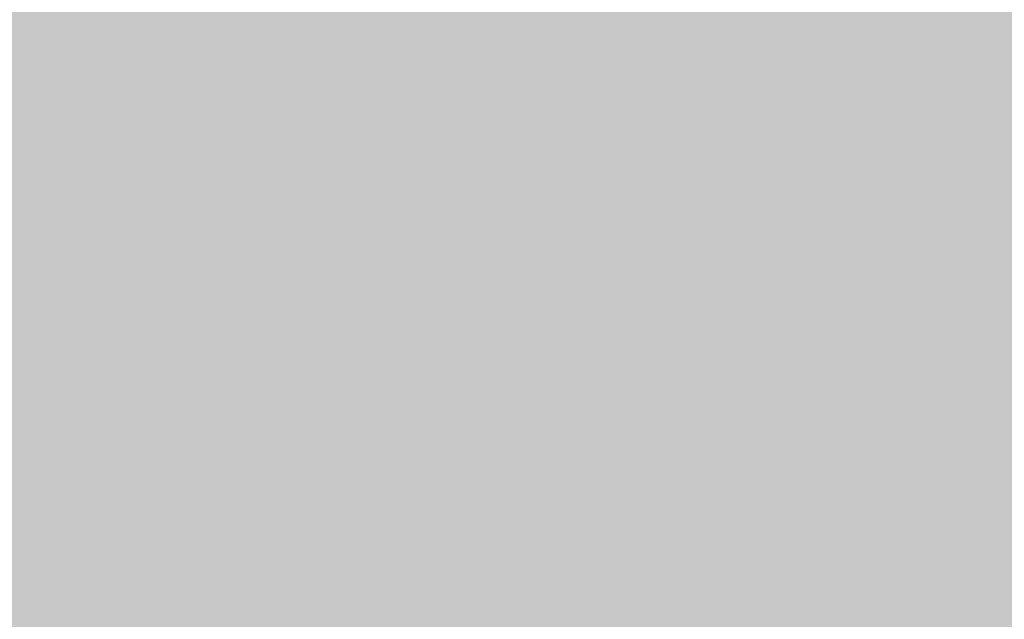
# Model space of a CAD drawing. Units: feet. Extents: x 3168 to 4724, y 827 to 1477.
# Tile 61 of 256: x 3273.145496 to 3273.147847, y 1099.01485 to 1099.016281. Entities that reach past the tile are written whole.
import ezdxf

# ---------------------------------------------------------------- set-up
doc = ezdxf.new("R2010")
doc.units = ezdxf.units.FT
doc.layers.add('A-ELEV', color=7, linetype='Continuous', lineweight=35)
doc.layers.add('A-ELEV-PATT', color=8, linetype='Continuous', lineweight=13)

msp = doc.modelspace()

# ---------------------------------------------------------------- hatches: boundary and pattern name
at = {"layer": 'A-ELEV-PATT'}
h = msp.add_hatch(color=256, dxfattribs=at)
h.dxf.hatch_style = 1
edge = h.paths.add_edge_path()
edge.add_ellipse((3552.9057615, 979.2201412), major_axis=(36.7449243, 0), ratio=0.4848484848, start_angle=0, end_angle=360)
edge = h.paths.add_edge_path()
edge.add_ellipse((3559.8916366, 929.2522824), major_axis=(36.7449243, 0), ratio=0.4848484848, start_angle=0, end_angle=360)
edge = h.paths.add_edge_path()
edge.add_line((3299.3168105, 1198.606081), (3479.9167135, 1198.606081))
edge.add_line((3479.9167135, 1198.606081), (3479.9167135, 1209.8685704))
edge.add_spline(control_points=[(3479.9167135, 1209.8685704), (3464.3011571, 1209.8685704), (3448.6856007, 1209.8685704), (3410.949139, 1209.8685704), (3388.8282339, 1209.8685704), (3355.6468761, 1209.8685704), (3344.5864235, 1209.8685704), (3327.9957446, 1209.8685704), (3322.4655183, 1209.8685704), (3314.1701788, 1209.8685704), (3311.4050657, 1209.8685704), (3307.257396, 1209.8685704), (3305.8748394, 1209.8685704), (3303.8010045, 1209.8685704), (3303.1097262, 1209.8685704), (3302.0728088, 1209.8685704), (3301.7271697, 1209.8685704), (3301.2087109, 1209.8685704), (3301.0358914, 1209.8685704), (3300.776662, 1209.8685704), (3300.6902522, 1209.8685704), (3300.5606376, 1209.8685704), (3300.5174327, 1209.8685704), (3300.4526253, 1209.8685704), (3300.4310229, 1209.8685704), (3300.3986192, 1209.8685704), (3300.387818, 1209.8685704), (3300.3662155, 1209.8685704), (3300.3456757, 1209.8685704), (3300.3455476, 1209.8685704), (3300.345505, 1209.8685704), (3300.3433041, 1209.8685704), (3300.341146, 1209.8685707), (3300.337909, 1209.8685714), (3300.33683, 1209.8685718), (3300.3339422, 1209.8685728), (3300.3321334, 1209.8685736), (3300.3255154, 1209.8685773), (3300.3207065, 1209.8685812), (3300.3109248, 1209.8685917), (3300.305952, 1209.8685984), (3300.2905113, 1209.8686233), (3300.2800452, 1209.8686461), (3300.2324255, 1209.868777), (3300.1952979, 1209.868954), (3299.9510684, 1209.8706077), (3299.7448244, 1209.8743259), (3299.4368271, 1209.8832566), (3299.3343894, 1209.8867924), (3299.181079, 1209.8929197), (3299.1300333, 1209.8950994), (3298.6522171, 1209.9168011), (3298.2294605, 1209.9457176), (3297.6016312, 1210.0023671), (3297.3934043, 1210.0234637), (3297.082652, 1210.058309), (3296.9793324, 1210.0704575), (3296.2929541, 1210.1548606), (3295.7181475, 1210.2433556), (3294.8687167, 1210.3988504), (3294.5876997, 1210.4544779), (3294.1693407, 1210.5433488), (3294.0304153, 1210.5738777), (3291.7071487, 1211.1012), (3289.6535901, 1211.8134353), (3285.7762586, 1213.5639876), (3283.9514101, 1214.6034778), (3280.512159, 1216.9800798), (3278.8972407, 1218.3175918), (3276.3799143, 1220.829489), (3275.4160415, 1221.9177379), (3274.0393421, 1223.7076996), (3273.5810428, 1224.3495346), (3273.1432283, 1225.0163162)], knot_values=[39.119033, 39.119033, 39.119033, 39.119033, 39.286353, 39.286353, 39.523379, 39.523379, 39.641892, 39.641892, 39.701148, 39.701148, 39.730777, 39.730777, 39.745591, 39.745591, 39.752998, 39.752998, 39.756701, 39.756701, 39.758553, 39.758553, 39.759479, 39.759479, 39.759942, 39.759942, 39.760173, 39.760173, 39.760289, 39.760289, 39.760405, 39.760405, 39.760463, 39.760463, 39.763389, 39.763389, 39.764851, 39.764851, 39.767304, 39.767304, 39.773825, 39.773825, 39.78057, 39.78057, 39.79477, 39.79477, 39.845194, 39.845194, 40.126715, 40.126715, 40.267476, 40.267476, 40.337856, 40.337856, 40.927023, 40.927023, 41.221606, 41.221606, 41.368898, 41.368898, 42.202622, 42.202622, 42.619485, 42.619485, 42.827916, 42.827916, 46.118323, 46.118323, 49.408731, 49.408731, 52.699139, 52.699139, 54.927489, 54.927489, 56.104228, 56.104228, 56.104228, 56.104228], weights=[1, 1, 1, 1, 1, 1, 1, 1, 1, 1, 1, 1, 1, 1, 1, 1, 1, 1, 1, 1, 1, 1, 1, 1, 1, 1, 1, 1, 1, 1, 1, 1, 1, 1, 1, 1, 1, 1, 1, 1, 1, 1, 1, 1, 1, 1, 1, 1, 1, 1, 1, 1, 1, 1, 1, 1, 1, 1, 1, 1, 1, 1, 1, 1, 1, 1, 1, 1, 1, 1, 1, 1, 1, 1], degree=3, periodic=0)
edge.add_line((3273.1432283, 1225.0163162), (3273.1432283, 1099.0163162))
edge.add_line((3273.1432283, 1099.0163162), (3299.3168105, 1099.0163162))
edge.add_line((3299.3168105, 1099.0163162), (3299.3168105, 1198.606081))
edge = h.paths.add_edge_path()
edge.add_line((3304.7584434, 1324.15806), (3479.9167135, 1324.15806))
edge.add_line((3479.9167135, 1324.15806), (3479.9167135, 1335.7146184))
edge.add_line((3479.9167135, 1335.7146184), (3269.1616284, 1335.7146184))
edge.add_spline(control_points=[(3269.1616284, 1335.7146184), (3264.0242315, 1335.7146184), (3258.364118, 1328.9581888), (3259.2643109, 1323.9002743)], knot_values=[0, 0, 0, 0, 15.412191, 15.412191, 15.412191, 15.412191], degree=3, periodic=0)
edge.add_line((3259.2643109, 1323.9002743), (3265.5168487, 1288.7691348))
edge.add_line((3265.5168487, 1288.7691348), (3275.2651026, 1261.5456259))
edge.add_line((3275.2651026, 1261.5456259), (3304.7584434, 1261.5456259))
edge.add_line((3304.7584434, 1261.5456259), (3304.7584434, 1324.15806))
h = msp.add_hatch(color=256, dxfattribs=at)
h.dxf.hatch_style = 1
h.paths.add_polyline_path([(3384.5252473, 1099.0163162), (3335.0291678, 1099.0163162), (3299.3168105, 1099.0163162), (3273.1432283, 1099.0163162), (3217.5653642, 1099.0163162), (3168.0692847, 827.1162598), (3335.0291678, 827.1162598)])

# ---------------------------------------------------------------- linework, layer by layer
at = {"layer": 'A-ELEV'}
msp.add_open_spline([(3808.5202001, 1099.0163162), (3808.5202001, 1141.413235), (3808.5202001, 1183.8101539), (3808.5202001, 1226.6353244), (3808.5202001, 1227.0635761), (3808.5202001, 1227.4918279), (3811.491871, 1248.9946729), (3814.463542, 1270.497518), (3817.4652299, 1292.2175635), (3817.4952467, 1292.434764), (3817.5252636, 1292.6519644), (3817.5728014, 1310.1067483), (3817.6203393, 1327.5615322), (3817.6678771, 1345.0163162), (3817.6678771, 1345.4579619), (3817.6678771, 1345.8996077), (3817.6678771, 1346.4560466), (3817.6678771, 1346.5708398), (3817.6678771, 1346.7528874), (3817.6678771, 1346.8201418), (3817.6678771, 1346.9348705), (3817.6678771, 1346.9823447), (3817.6678771, 1347.0385872), (3817.6678771, 1347.0473556), (3817.6678771, 1347.0736607), (3817.667877, 1347.0593025), (3817.6678766, 1347.0615455), (3817.6678764, 1347.0626669), (3817.6678754, 1347.0660311), (3817.6678743, 1347.0682738), (3817.6678701, 1347.0750012), (3817.667866, 1347.0794856), (3817.6678493, 1347.0929368), (3817.6678325, 1347.1019019), (3817.6677657, 1347.1287896), (3817.6676988, 1347.1467049), (3817.6674317, 1347.2004211), (3817.6671649, 1347.2361922), (3817.6661003, 1347.3433849), (3817.6650383, 1347.4146859), (3817.6608124, 1347.6280949), (3817.6566084, 1347.7697085), (3817.6399698, 1348.1924868), (3817.6235091, 1348.4715855), (3817.5590944, 1349.3000666), (3817.4961208, 1349.8405878), (3817.2554319, 1351.4241561), (3817.0263177, 1352.4287852), (3816.3068713, 1354.8889138), (3815.7437452, 1356.2687272), (3814.4639586, 1358.8192105), (3813.7464132, 1359.9909676), (3812.1958378, 1362.1723433), (3811.3622453, 1363.1821237), (3809.5888357, 1365.0690087), (3808.6488164, 1365.9461052), (3806.6542623, 1367.5796162), (3805.5997024, 1368.336154), (3803.3528906, 1369.7223272), (3802.1605354, 1370.352386), (3799.6008131, 1371.4535864), (3798.2326878, 1371.9254812), (3795.2800838, 1372.6346239), (3793.6931479, 1372.8720685), (3791.8694413, 1372.9264797), (3791.7408615, 1372.9292203), (3791.3533713, 1372.9341014), (3791.0927074, 1372.9329013), (3790.3041163, 1372.9150676), (3789.7695426, 1372.8841946), (3789.20919, 1372.8302363), (3789.1906217, 1372.8284241), (3789.1348916, 1372.8229123), (3789.097705, 1372.8191375), (3789.0484446, 1372.8140077), (3789.0364001, 1372.8127432), (3789.0002562, 1372.808918), (3788.9761468, 1372.8063255), (3788.9494049, 1372.8034042), (3788.9467858, 1372.8031177), (3788.9425667, 1372.8026552), (3788.9409669, 1372.8024797), (3788.9385718, 1372.8022166), (3788.9377765, 1372.8021292), (3788.9353908, 1372.8018669), (3788.8675349, 1372.7944024), (3788.7568665, 1372.7822285), (3788.7015323, 1372.7761415), (3788.5355297, 1372.7578805), (3788.4248612, 1372.7457065), (3788.092856, 1372.7091846), (3787.8715192, 1372.6848366), (3787.2075086, 1372.6117927), (3786.764835, 1372.5630968), (3785.436814, 1372.417009), (3784.5514666, 1372.3196171), (3781.8954246, 1372.0274416), (3780.1247299, 1371.8326579), (3774.8126458, 1371.2483067), (3771.2712564, 1370.8587393), (3760.6470883, 1369.6900371), (3753.5643095, 1368.9109022), (3732.3159732, 1366.5734977), (3718.1504157, 1365.015228), (3694.0067577, 1362.3593262), (3684.0286573, 1361.2616941), (3674.0505568, 1360.1640619), (3664.6006617, 1360.1640619), (3655.1507666, 1360.1640619), (3626.8010812, 1360.1640619), (3607.9012909, 1360.1640619), (3551.2019201, 1360.1640619), (3513.4023395, 1360.1640619), (3467.7251817, 1360.1640619), (3459.8476045, 1360.1640619), (3436.2148727, 1360.1640619), (3420.4597182, 1360.1640619), (3373.1942547, 1360.1640619), (3341.6839457, 1360.1640619), (3302.8481616, 1360.1640619), (3295.5226865, 1360.1640619), (3286.0382916, 1360.1640619), (3283.8793719, 1360.1640619), (3277.4026128, 1360.1640619), (3273.0847733, 1360.1640619), (3267.7328511, 1360.1640619), (3266.6987684, 1360.1640619), (3263.5965201, 1360.1640619), (3261.5283546, 1360.1640619), (3259.2369429, 1360.1640619), (3259.0136967, 1360.1640619), (3258.3439582, 1360.1640619), (3257.8974658, 1360.1640619), (3257.4309979, 1360.1640619), (3257.4110224, 1360.1640619), (3257.3705735, 1360.1640619), (3257.3754695, 1360.1640619), (3257.3745975, 1360.1640619), (3257.3739371, 1360.1640618), (3257.3719559, 1360.1640616), (3257.3706351, 1360.1640613), (3257.366673, 1360.16406), (3257.3640318, 1360.1640586), (3257.3561088, 1360.1640529), (3257.3508277, 1360.1640469), (3257.3349869, 1360.1640226), (3257.3244299, 1360.163998), (3257.2927692, 1360.1638987), (3257.2716761, 1360.1637987), (3257.208439, 1360.1633975), (3257.1663373, 1360.1629953), (3257.0402058, 1360.1613882), (3256.9563493, 1360.1597827), (3256.705504, 1360.1533932), (3256.53924, 1360.1470361), (3256.0435702, 1360.1219156), (3255.717296, 1360.0971018), (3254.7524458, 1360.0004808), (3254.1279679, 1359.906513), (3252.1800666, 1359.5253322), (3250.9415739, 1359.1439911), (3248.6701751, 1358.2432905), (3247.6357388, 1357.7238339), (3245.7326321, 1356.6034712), (3244.8633884, 1356.0020595), (3243.2531076, 1354.7428655), (3242.511972, 1354.0847309), (3240.7510518, 1352.3447812), (3239.8009609, 1351.229574), (3238.0877694, 1348.8724402), (3237.3246853, 1347.6303552), (3235.9825098, 1344.9716321), (3235.4022051, 1343.554907), (3234.5910812, 1340.8154577), (3234.3108819, 1339.5435498), (3233.9764902, 1336.8025605), (3233.9221126, 1335.3308771), (3234.1489156, 1332.5912693), (3234.3495287, 1331.3672011), (3234.7198926, 1329.9993668), (3234.7524228, 1329.8833616), (3234.853619, 1329.5347966), (3234.9258923, 1329.301685), (3235.0248359, 1329.0025524), (3235.0469235, 1328.936928), (3235.0776388, 1328.8472393), (3235.0859239, 1328.8231979), (3235.1109389, 1328.7510642), (3235.1278282, 1328.7029624), (3235.1479919, 1328.6462418), (3235.1510592, 1328.6376324), (3235.1560959, 1328.6235265), (3235.1580611, 1328.6180301), (3235.1602094, 1328.6120302), (3235.1656119, 1328.596943), (3235.1800989, 1328.556486), (3235.190263, 1328.5281009), (3235.2207556, 1328.4429457), (3235.241084, 1328.3861755), (3235.3020692, 1328.215865), (3235.3427259, 1328.1023247), (3235.4646962, 1327.7617038), (3235.5460097, 1327.5346232), (3235.7899503, 1326.8533813), (3235.9525774, 1326.39922), (3236.4404586, 1325.0367362), (3236.7657127, 1324.1284137), (3237.7414751, 1321.4034462), (3238.3919833, 1319.5868011), (3240.3435081, 1314.136866), (3241.6445245, 1310.503576), (3245.547574, 1299.6037058), (3248.149607, 1292.3371257), (3255.955706, 1270.5373853), (3261.1597719, 1256.004225), (3267.3876177, 1238.6120011), (3268.4113975, 1235.7529374), (3269.5103781, 1232.6838639), (3269.5855789, 1232.473854), (3269.7066118, 1232.1358507), (3269.752444, 1232.0078573), (3269.8273289, 1231.7987296), (3269.8563817, 1231.7175953), (3269.9063247, 1231.5781217), (3269.927215, 1231.5197823), (3269.9724682, 1231.3934057), (3269.9968311, 1231.3253685), (3270.0265026, 1231.2425062), (3270.0318112, 1231.2276812), (3270.0402823, 1231.2040243), (3270.0392242, 1231.2069792), (3270.0393595, 1231.2066014), (3270.0394271, 1231.2064125), (3270.0396301, 1231.2058458), (3270.0397654, 1231.205468), (3270.0401713, 1231.2043346), (3270.040442, 1231.2035791), (3270.041254, 1231.2013125), (3270.0417955, 1231.1998016), (3270.0434203, 1231.195269), (3270.044504, 1231.1922477), (3270.0477563, 1231.1831849), (3270.0499263, 1231.1771446), (3270.0564418, 1231.1590283), (3270.0607927, 1231.146957), (3270.0738674, 1231.1107614), (3270.0826128, 1231.0866558), (3270.1089357, 1231.0144129), (3270.1265997, 1230.9663498), (3270.1799341, 1230.8224568), (3270.2159467, 1230.7269233), (3270.3253234, 1230.4415078), (3270.4000257, 1230.2528107), (3270.6292491, 1229.6914436), (3270.7888829, 1229.3235005), (3271.2864875, 1228.2383194), (3271.6430996, 1227.5397546), (3272.7758592, 1225.515277), (3273.6141694, 1224.2605021), (3275.4160415, 1221.9177379), (3276.3799143, 1220.829489), (3278.8972407, 1218.3175918), (3280.512159, 1216.9800798), (3283.9514101, 1214.6034778), (3285.7762586, 1213.5639876), (3289.6535901, 1211.8134353), (3291.7071487, 1211.1012), (3294.0304153, 1210.5738777), (3294.1693407, 1210.5433488), (3294.5876997, 1210.4544779), (3294.8687167, 1210.3988504), (3295.7181475, 1210.2433556), (3296.2929541, 1210.1548606), (3296.9793324, 1210.0704575), (3297.082652, 1210.058309), (3297.3934043, 1210.0234637), (3297.6016312, 1210.0023671), (3298.2294605, 1209.9457176), (3298.6522171, 1209.9168011), (3299.1300333, 1209.8950994), (3299.181079, 1209.8929197), (3299.3343894, 1209.8867924), (3299.4368271, 1209.8832566), (3299.7448244, 1209.8743259), (3299.9510684, 1209.8706077), (3300.1952979, 1209.868954), (3300.2324255, 1209.868777), (3300.2800452, 1209.8686461), (3300.2905113, 1209.8686233), (3300.305952, 1209.8685984), (3300.3109248, 1209.8685917), (3300.3207065, 1209.8685812), (3300.3255154, 1209.8685773), (3300.3321334, 1209.8685736), (3300.3339422, 1209.8685728), (3300.33683, 1209.8685718), (3300.337909, 1209.8685714), (3300.341146, 1209.8685707), (3300.3433041, 1209.8685704), (3300.345505, 1209.8685704), (3300.3455476, 1209.8685704), (3300.3456757, 1209.8685704), (3300.3662155, 1209.8685704), (3300.387818, 1209.8685704), (3300.3986192, 1209.8685704), (3300.4310229, 1209.8685704), (3300.4526253, 1209.8685704), (3300.5174327, 1209.8685704), (3300.5606376, 1209.8685704), (3300.6902522, 1209.8685704), (3300.776662, 1209.8685704), (3301.0358914, 1209.8685704), (3301.2087109, 1209.8685704), (3301.7271697, 1209.8685704), (3302.0728088, 1209.8685704), (3303.1097262, 1209.8685704), (3303.8010045, 1209.8685704), (3305.8748394, 1209.8685704), (3307.257396, 1209.8685704), (3311.4050657, 1209.8685704), (3314.1701788, 1209.8685704), (3322.4655183, 1209.8685704), (3327.9957446, 1209.8685704), (3344.5864235, 1209.8685704), (3355.6468761, 1209.8685704), (3388.8282339, 1209.8685704), (3410.949139, 1209.8685704), (3477.3118546, 1209.8685704), (3521.553665, 1209.8685704), (3566.8361836, 1209.8685704), (3567.8768919, 1209.8685704), (3570.9990167, 1209.8685704), (3573.0804332, 1209.8685704), (3575.7813964, 1209.8685704), (3576.4009432, 1209.8685704), (3577.2958211, 1209.8685704), (3577.5711523, 1209.8685704), (3578.3971458, 1209.8685704), (3578.9478081, 1209.8685704), (3579.7564907, 1209.8685704), (3580.0145108, 1209.8685704), (3580.3427367, 1209.8685704), (3580.3268649, 1209.8685704), (3580.3271702, 1209.8685704), (3580.3273229, 1209.8685704), (3580.3277809, 1209.8685704), (3580.3280863, 1209.8685704), (3580.3290024, 1209.8685703), (3580.3296132, 1209.8685702), (3580.3314455, 1209.8685699), (3580.332667, 1209.8685697), (3580.336332, 1209.8685685), (3580.3387755, 1209.8685674), (3580.3461066, 1209.8685629), (3580.350995, 1209.8685584), (3580.3656627, 1209.8685402), (3580.3754446, 1209.868522), (3580.4048012, 1209.8684493), (3580.4243863, 1209.8683764), (3580.4831833, 1209.8680848), (3580.5224371, 1209.8677929), (3580.6403612, 1209.8666242), (3580.7191947, 1209.8654543), (3580.9563152, 1209.8607663), (3581.1152222, 1209.85607), (3581.5941635, 1209.8372298), (3581.9164188, 1209.8183314), (3582.8899466, 1209.7424284), (3583.547986, 1209.6661692), (3585.5318268, 1209.3606172), (3586.8672159, 1209.0538859), (3589.4715454, 1208.2524717), (3590.7402412, 1207.7578521), (3591.9954511, 1207.1588024), (3592.057809, 1207.1287398), (3592.2442418, 1207.0379536), (3592.3676757, 1206.9766317), (3592.73528, 1206.7903591), (3592.9767518, 1206.663101), (3593.2445387, 1206.5164414), (3593.2747313, 1206.4998248), (3593.3651153, 1206.4498388), (3593.4251129, 1206.4163333), (3593.6043138, 1206.3152851), (3593.7227254, 1206.2472105), (3593.8572122, 1206.1683978), (3593.8743621, 1206.1583193), (3593.925741, 1206.1280407), (3593.9598989, 1206.1077976), (3594.0620855, 1206.0468991), (3594.1298272, 1206.0060745), (3594.2084359, 1205.9581709), (3594.2196829, 1205.9513043), (3594.253391, 1205.9306863), (3594.2758193, 1205.9169166), (3594.3429716, 1205.8755358), (3594.3875633, 1205.8478526), (3594.4336161, 1205.8190499), (3594.4352559, 1205.818024), (3594.4401746, 1205.8149461), (3594.4434527, 1205.8128936), (3594.4471229, 1205.8105944), (3594.4475159, 1205.8103482), (3594.4486949, 1205.8096095), (3594.4494808, 1205.8091171), (3594.4503663, 1205.8085621), (3594.4504658, 1205.8084998), (3594.4506003, 1205.8084155), (3594.4673993, 1205.7978872), (3594.4932689, 1205.7816741), (3594.5062037, 1205.7735675), (3594.5450081, 1205.7492479), (3594.5708778, 1205.7330348), (3594.6484866, 1205.6843956), (3594.7002258, 1205.6519694), (3594.8554436, 1205.5546909), (3594.958922, 1205.4898386), (3595.2693574, 1205.2952816), (3595.4763144, 1205.1655769), (3596.0971852, 1204.7764629), (3596.5110991, 1204.5170536), (3597.7528407, 1203.7388256), (3598.5806685, 1203.220007), (3601.0641518, 1201.663551), (3602.7198073, 1200.6259137), (3607.686774, 1197.5130018), (3610.998085, 1195.4377272), (3620.9320182, 1189.2119034), (3627.5546404, 1185.0613542), (3647.4225068, 1172.6097066), (3660.6677511, 1164.3086082), (3700.403484, 1139.405313), (3726.8939725, 1122.8031161), (3757.2057154, 1103.8060516), (3761.0269697, 1101.4111839), (3764.848224, 1099.0163162), (3745.3282713, 1099.0163162), (3725.8083186, 1099.0163162), (3706.288366, 1099.0163162), (3706.288366, 1108.4532371), (3706.288366, 1117.890158), (3706.288366, 1127.3270789), (3710.7507544, 1127.3270789), (3715.2131428, 1127.3270789), (3719.6755312, 1127.3270789)], degree=3, knots=[0, 0, 0, 0, 0.982037, 0.982037, 0.991957, 0.991957, 0.991957, 1.966522, 1.966522, 1.976367, 1.976367, 1.976367, 2.976367, 2.976367, 2.976367, 3.00169, 3.00169, 3.008272, 3.008272, 3.012129, 3.012129, 3.014851, 3.014851, 3.015353, 3.015353, 3.016359, 3.016359, 3.017365, 3.017365, 3.019376, 3.019376, 3.023398, 3.023398, 3.031442, 3.031442, 3.047531, 3.047531, 3.079708, 3.079708, 3.144063, 3.144063, 3.272772, 3.272772, 3.53019, 3.53019, 4.045026, 4.045026, 5.074698, 5.074698, 6.700878, 6.700878, 8.327058, 8.327058, 9.953238, 9.953238, 11.579418, 11.579418, 13.205598, 13.205598, 14.831778, 14.831778, 16.457958, 16.457958, 18.084138, 18.084138, 18.206872, 18.206872, 18.45234, 18.45234, 18.943275, 18.943275, 18.960093, 18.960093, 18.993729, 18.993729, 19.00461, 19.00461, 19.026374, 19.026374, 19.028737, 19.028737, 19.03018, 19.03018, 19.030897, 19.030897, 19.032332, 19.032332, 19.033766, 19.033766, 19.036636, 19.036636, 19.042374, 19.042374, 19.053851, 19.053851, 19.076805, 19.076805, 19.122714, 19.122714, 19.21453, 19.21453, 19.398163, 19.398163, 19.765429, 19.765429, 20.024128, 20.024128, 20.024128, 20.092031, 20.092031, 20.227836, 20.227836, 20.499446, 20.499446, 20.556051, 20.556051, 20.66926, 20.66926, 20.895678, 20.895678, 20.948316, 20.948316, 20.963829, 20.963829, 20.994855, 20.994855, 21.002285, 21.002285, 21.017146, 21.017146, 21.01875, 21.01875, 21.021959, 21.021959, 21.022102, 21.022102, 21.022249, 21.022249, 21.022708, 21.022708, 21.023627, 21.023627, 21.025464, 21.025464, 21.029138, 21.029138, 21.036486, 21.036486, 21.051183, 21.051183, 21.080575, 21.080575, 21.139361, 21.139361, 21.256932, 21.256932, 21.492073, 21.492073, 21.962356, 21.962356, 23.01002, 23.01002, 24.057684, 24.057684, 25.105348, 25.105348, 26.153011, 26.153011, 27.776787, 27.776787, 29.400562, 29.400562, 31.024337, 31.024337, 32.278801, 32.278801, 33.533265, 33.533265, 34.467568, 34.467568, 34.553971, 34.553971, 34.726776, 34.726776, 34.775309, 34.775309, 34.793079, 34.793079, 34.82862, 34.82862, 34.834979, 34.834979, 34.839039, 34.839039, 34.839411, 34.839411, 34.840285, 34.840285, 34.842034, 34.842034, 34.845531, 34.845531, 34.852525, 34.852525, 34.866512, 34.866512, 34.894488, 34.894488, 34.950439, 34.950439, 35.062342, 35.062342, 35.286147, 35.286147, 35.733758, 35.733758, 35.821815, 35.821815, 35.828283, 35.828283, 35.832225, 35.832225, 35.834724, 35.834724, 35.836521, 35.836521, 35.838617, 35.838617, 35.839073, 35.839073, 35.839345, 35.839345, 35.839617, 35.839617, 35.840161, 35.840161, 35.841249, 35.841249, 35.843425, 35.843425, 35.847778, 35.847778, 35.856482, 35.856482, 35.873891, 35.873891, 35.908709, 35.908709, 35.978345, 35.978345, 36.117617, 36.117617, 36.396161, 36.396161, 36.953248, 36.953248, 38.067423, 38.067423, 40.295772, 40.295772, 42.524122, 42.524122, 45.81453, 45.81453, 49.104937, 49.104937, 52.395345, 52.395345, 52.603776, 52.603776, 53.020639, 53.020639, 53.854363, 53.854363, 54.001655, 54.001655, 54.296238, 54.296238, 54.885405, 54.885405, 54.955785, 54.955785, 55.096546, 55.096546, 55.378067, 55.378067, 55.42849, 55.42849, 55.442691, 55.442691, 55.449436, 55.449436, 55.455957, 55.455957, 55.458409, 55.458409, 55.459872, 55.459872, 55.462798, 55.462798, 55.462856, 55.462856, 55.462972, 55.462972, 55.463088, 55.463088, 55.463319, 55.463319, 55.463782, 55.463782, 55.464708, 55.464708, 55.46656, 55.46656, 55.470263, 55.470263, 55.47767, 55.47767, 55.492484, 55.492484, 55.522112, 55.522112, 55.581369, 55.581369, 55.699882, 55.699882, 55.936907, 55.936907, 56.410959, 56.410959, 56.42211, 56.42211, 56.444413, 56.444413, 56.451051, 56.451051, 56.454001, 56.454001, 56.459901, 56.459901, 56.462666, 56.462666, 56.463418, 56.463418, 56.464171, 56.464171, 56.465675, 56.465675, 56.468684, 56.468684, 56.474702, 56.474702, 56.486738, 56.486738, 56.51081, 56.51081, 56.558955, 56.558955, 56.655243, 56.655243, 56.847821, 56.847821, 57.232975, 57.232975, 58.003284, 58.003284, 59.543901, 59.543901, 62.625137, 62.625137, 68.787607, 68.787607, 74.950078, 74.950078, 75.27336, 75.27336, 75.919923, 75.919923, 77.213051, 77.213051, 77.377769, 77.377769, 77.707206, 77.707206, 78.366079, 78.366079, 78.462532, 78.462532, 78.655436, 78.655436, 79.041245, 79.041245, 79.105735, 79.105735, 79.234714, 79.234714, 79.492672, 79.492672, 79.502197, 79.502197, 79.521249, 79.521249, 79.523534, 79.523534, 79.528103, 79.528103, 79.528682, 79.528682, 79.528885, 79.528885, 79.529089, 79.529089, 79.529495, 79.529495, 79.530308, 79.530308, 79.531935, 79.531935, 79.535187, 79.535187, 79.541693, 79.541693, 79.554704, 79.554704, 79.580725, 79.580725, 79.632769, 79.632769, 79.736856, 79.736856, 79.94503, 79.94503, 80.361377, 80.361377, 80.421435, 80.421435, 80.421435, 81.421435, 81.421435, 81.421435, 82.421435, 82.421435, 82.421435, 83.421435, 83.421435, 83.421435, 83.421435], dxfattribs=at)

doc.saveas('drawing.dxf')
